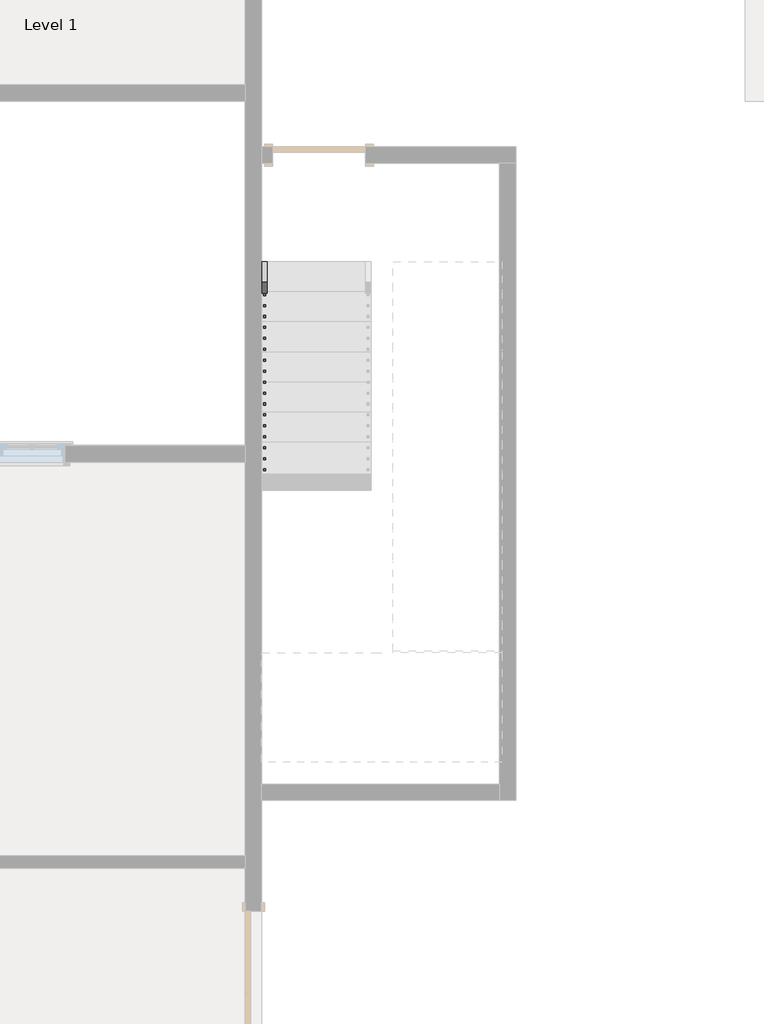
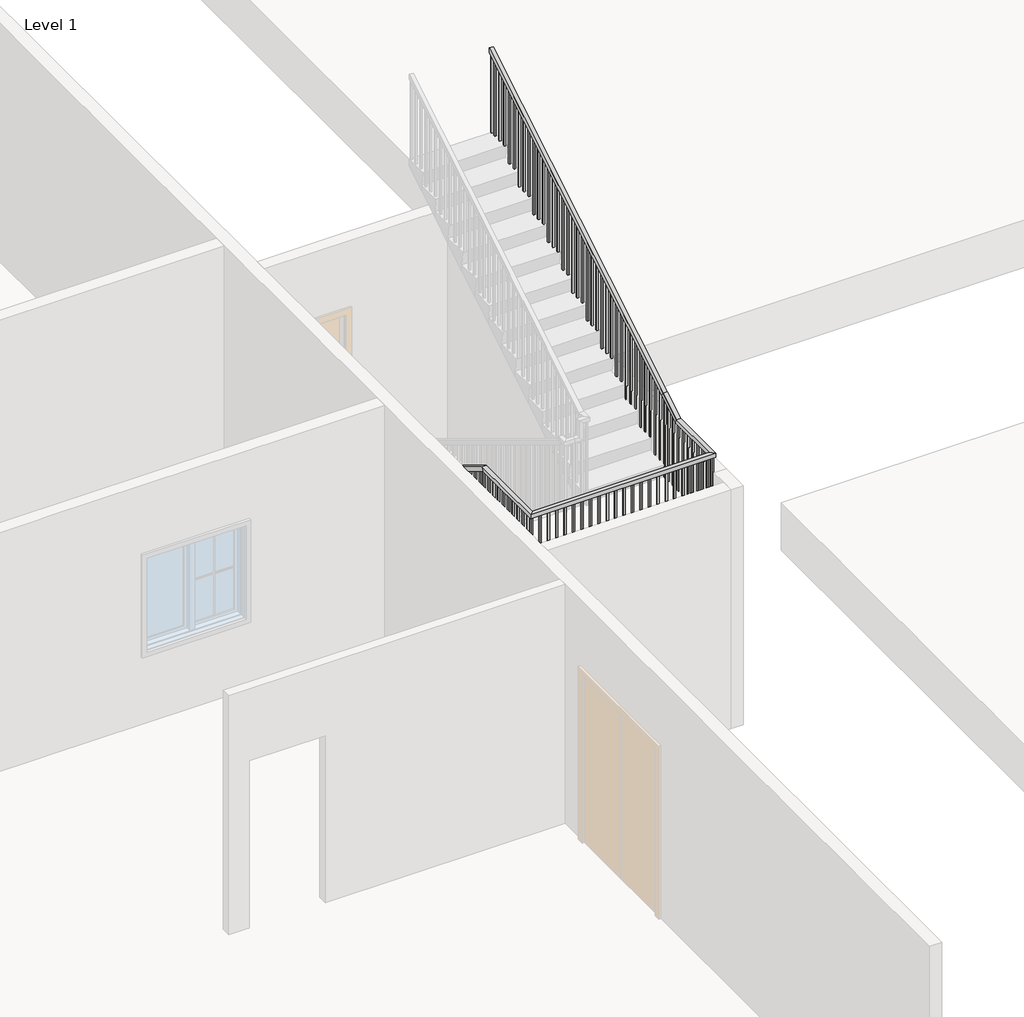
# One storey, part 4 of 7: 1 railing.
"""IFC4 building model written with IfcOpenShell, lengths in millimetres."""

from ifc_helpers import new_model, si_unit, frame, origin, place, context, project, spatial, polyline, outline, extrude, faceted_brep, element, save

model = new_model("IFC4")

# Units and contexts
model_context = context("Model", 3, world=origin())
ifc_project = project(units=[si_unit("LENGTHUNIT", "METRE", prefix="MILLI")], contexts=[model_context])

# Site, building, storey
site = spatial("IfcSite", under=ifc_project)
building = spatial("IfcBuilding", under=site)
storey = spatial("IfcBuildingStorey", under=building, Name="Level 1", Elevation=0.0)

# Railing
placement = place(None, origin())
element("IfcRailing", 1, ObjectType="Handrail - Rectangular", at=placement, inside=storey, context=model_context, shape_type="SolidModel", body=[
    faceted_brep([(-3452.3844485, 646.3269271, 1083.7333333), (-3452.3844485, 646.3269271, 1024.3318731), (-3503.1844485, 646.3269271, 1024.3318731), (-3503.1844485, 646.3269271, 1083.7333333), (-3452.3844485, -2985.8730729, 3285.0666667), (-3452.3844485, -3000.0654823, 3234.2666667), (-3503.1844485, -3000.0654823, 3234.2666667), (-3503.1844485, -2985.8730729, 3285.0666667), (-3452.3844485, -3951.0730729, 3285.0666667), (-3452.3844485, -3951.0730729, 3234.2666667), (-3503.1844485, -4001.8730729, 3234.2666667), (-3503.1844485, -4001.8730729, 3285.0666667), (-1318.7844485, -3951.0730729, 3285.0666667), (-1318.7844485, -3951.0730729, 3234.2666667), (-1267.9844485, -4001.8730729, 3234.2666667), (-1267.9844485, -4001.8730729, 3285.0666667), (-1318.7844485, -3265.2730729, 3285.0666667), (-1318.7844485, -3251.0806634, 3234.2666667), (-1267.9844485, -3251.0806634, 3234.2666667), (-1267.9844485, -3265.2730729, 3285.0666667), (-1318.7844485, -2985.8730729, 3454.4), (-1318.7844485, -2959.5433457, 3410.9559502), (-1267.9844485, -2959.5433457, 3410.9559502), (-1267.9844485, -2985.8730729, 3454.4), (-1318.7844485, 646.3269271, 5655.7333333), (-1267.9844485, 646.3269271, 5655.7333333), (-1267.9844485, 646.3269271, 5596.3318731), (-1318.7844485, 646.3269271, 5596.3318731)], [[[0, 1, 2, 3]], [[1, 0, 4, 5]], [[2, 1, 5, 6]], [[3, 2, 6, 7]], [[0, 3, 7, 4]], [[5, 4, 8, 9]], [[6, 5, 9, 10]], [[7, 6, 10, 11]], [[4, 7, 11, 8]], [[9, 8, 12, 13]], [[10, 9, 13, 14]], [[11, 10, 14, 15]], [[8, 11, 15, 12]], [[13, 12, 16, 17]], [[14, 13, 17, 18]], [[15, 14, 18, 19]], [[12, 15, 19, 16]], [[17, 16, 20, 21]], [[18, 17, 21, 22]], [[19, 18, 22, 23]], [[16, 19, 23, 20]], [[24, 25, 26, 27]], [[21, 20, 24, 27]], [[22, 21, 27, 26]], [[23, 22, 26, 25]], [[20, 23, 25, 24]]]),
    extrude(outline(polyline([(560.6019271, 5544.3773276), (579.6519271, 5555.9227822), (579.6519271, 4572.0), (560.6019271, 4572.0), (560.6019271, 5544.3773276)])), frame((-1302.9094485, 0.0, 0.0), z_axis=(1.0, 0.0, 0.0), x_axis=(0.0, 1.0, 0.0)), (0.0, 0.0, 1.0), 19.05),
    extrude(outline(polyline([(459.0019271, 5482.80157), (478.0519271, 5494.3470246), (478.0519271, 4572.0), (459.0019271, 4572.0), (459.0019271, 5482.80157)])), frame((-1302.9094485, 0.0, 0.0), z_axis=(1.0, 0.0, 0.0), x_axis=(0.0, 1.0, 0.0)), (0.0, 0.0, 1.0), 19.05),
    extrude(outline(polyline([(357.4019271, 5421.2258125), (376.4519271, 5432.771267), (376.4519271, 4572.0), (357.4019271, 4572.0), (357.4019271, 5421.2258125)])), frame((-1302.9094485, 0.0, 0.0), z_axis=(1.0, 0.0, 0.0), x_axis=(0.0, 1.0, 0.0)), (0.0, 0.0, 1.0), 19.05),
    extrude(outline(polyline([(255.8019271, 5359.6500549), (274.8519271, 5371.1955094), (274.8519271, 4402.6666667), (255.8019271, 4402.6666667), (255.8019271, 5359.6500549)])), frame((-1302.9094485, 0.0, 0.0), z_axis=(1.0, 0.0, 0.0), x_axis=(0.0, 1.0, 0.0)), (0.0, 0.0, 1.0), 19.05),
    extrude(outline(polyline([(154.2019271, 5298.0742973), (173.2519271, 5309.6197519), (173.2519271, 4402.6666667), (154.2019271, 4402.6666667), (154.2019271, 5298.0742973)])), frame((-1302.9094485, 0.0, 0.0), z_axis=(1.0, 0.0, 0.0), x_axis=(0.0, 1.0, 0.0)), (0.0, 0.0, 1.0), 19.05),
    extrude(outline(polyline([(52.6019271, 5236.4985397), (71.6519271, 5248.0439943), (71.6519271, 4233.3333333), (52.6019271, 4233.3333333), (52.6019271, 5236.4985397)])), frame((-1302.9094485, 0.0, 0.0), z_axis=(1.0, 0.0, 0.0), x_axis=(0.0, 1.0, 0.0)), (0.0, 0.0, 1.0), 19.05),
    extrude(outline(polyline([(-48.9980729, 5174.9227822), (-29.9480729, 5186.4682367), (-29.9480729, 4233.3333333), (-48.9980729, 4233.3333333), (-48.9980729, 5174.9227822)])), frame((-1302.9094485, 0.0, 0.0), z_axis=(1.0, 0.0, 0.0), x_axis=(0.0, 1.0, 0.0)), (0.0, 0.0, 1.0), 19.05),
    extrude(outline(polyline([(-150.5980729, 5113.3470246), (-131.5480729, 5124.8924791), (-131.5480729, 4233.3333333), (-150.5980729, 4233.3333333), (-150.5980729, 5113.3470246)])), frame((-1302.9094485, 0.0, 0.0), z_axis=(1.0, 0.0, 0.0), x_axis=(0.0, 1.0, 0.0)), (0.0, 0.0, 1.0), 19.05),
    extrude(outline(polyline([(-252.1980729, 5051.771267), (-233.1480729, 5063.3167216), (-233.1480729, 4064.0), (-252.1980729, 4064.0), (-252.1980729, 5051.771267)])), frame((-1302.9094485, 0.0, 0.0), z_axis=(1.0, 0.0, 0.0), x_axis=(0.0, 1.0, 0.0)), (0.0, 0.0, 1.0), 19.05),
    extrude(outline(polyline([(-353.7980729, 4990.1955094), (-334.7480729, 5001.740964), (-334.7480729, 4064.0), (-353.7980729, 4064.0), (-353.7980729, 4990.1955094)])), frame((-1302.9094485, 0.0, 0.0), z_axis=(1.0, 0.0, 0.0), x_axis=(0.0, 1.0, 0.0)), (0.0, 0.0, 1.0), 19.05),
    extrude(outline(polyline([(-455.3980729, 4928.6197519), (-436.3480729, 4940.1652064), (-436.3480729, 4064.0), (-455.3980729, 4064.0), (-455.3980729, 4928.6197519)])), frame((-1302.9094485, 0.0, 0.0), z_axis=(1.0, 0.0, 0.0), x_axis=(0.0, 1.0, 0.0)), (0.0, 0.0, 1.0), 19.05),
    extrude(outline(polyline([(-556.9980729, 4867.0439943), (-537.9480729, 4878.5894488), (-537.9480729, 3894.6666667), (-556.9980729, 3894.6666667), (-556.9980729, 4867.0439943)])), frame((-1302.9094485, 0.0, 0.0), z_axis=(1.0, 0.0, 0.0), x_axis=(0.0, 1.0, 0.0)), (0.0, 0.0, 1.0), 19.05),
    extrude(outline(polyline([(-658.5980729, 4805.4682367), (-639.5480729, 4817.0136913), (-639.5480729, 3894.6666667), (-658.5980729, 3894.6666667), (-658.5980729, 4805.4682367)])), frame((-1302.9094485, 0.0, 0.0), z_axis=(1.0, 0.0, 0.0), x_axis=(0.0, 1.0, 0.0)), (0.0, 0.0, 1.0), 19.05),
    extrude(outline(polyline([(-760.1980729, 4743.8924791), (-741.1480729, 4755.4379337), (-741.1480729, 3894.6666667), (-760.1980729, 3894.6666667), (-760.1980729, 4743.8924791)])), frame((-1302.9094485, 0.0, 0.0), z_axis=(1.0, 0.0, 0.0), x_axis=(0.0, 1.0, 0.0)), (0.0, 0.0, 1.0), 19.05),
    extrude(outline(polyline([(-861.7980729, 4682.3167216), (-842.7480729, 4693.8621761), (-842.7480729, 3725.3333333), (-861.7980729, 3725.3333333), (-861.7980729, 4682.3167216)])), frame((-1302.9094485, 0.0, 0.0), z_axis=(1.0, 0.0, 0.0), x_axis=(0.0, 1.0, 0.0)), (0.0, 0.0, 1.0), 19.05),
    extrude(outline(polyline([(-963.3980729, 4620.740964), (-944.3480729, 4632.2864185), (-944.3480729, 3725.3333333), (-963.3980729, 3725.3333333), (-963.3980729, 4620.740964)])), frame((-1302.9094485, 0.0, 0.0), z_axis=(1.0, 0.0, 0.0), x_axis=(0.0, 1.0, 0.0)), (0.0, 0.0, 1.0), 19.05),
    extrude(outline(polyline([(-1064.9980729, 4559.1652064), (-1045.9480729, 4570.710661), (-1045.9480729, 3556.0), (-1064.9980729, 3556.0), (-1064.9980729, 4559.1652064)])), frame((-1302.9094485, 0.0, 0.0), z_axis=(1.0, 0.0, 0.0), x_axis=(0.0, 1.0, 0.0)), (0.0, 0.0, 1.0), 19.05),
    extrude(outline(polyline([(-1166.5980729, 4497.5894488), (-1147.5480729, 4509.1349034), (-1147.5480729, 3556.0), (-1166.5980729, 3556.0), (-1166.5980729, 4497.5894488)])), frame((-1302.9094485, 0.0, 0.0), z_axis=(1.0, 0.0, 0.0), x_axis=(0.0, 1.0, 0.0)), (0.0, 0.0, 1.0), 19.05),
    extrude(outline(polyline([(-1268.1980729, 4436.0136913), (-1249.1480729, 4447.5591458), (-1249.1480729, 3556.0), (-1268.1980729, 3556.0), (-1268.1980729, 4436.0136913)])), frame((-1302.9094485, 0.0, 0.0), z_axis=(1.0, 0.0, 0.0), x_axis=(0.0, 1.0, 0.0)), (0.0, 0.0, 1.0), 19.05),
    extrude(outline(polyline([(-1369.7980729, 4374.4379337), (-1350.7480729, 4385.9833882), (-1350.7480729, 3386.6666667), (-1369.7980729, 3386.6666667), (-1369.7980729, 4374.4379337)])), frame((-1302.9094485, 0.0, 0.0), z_axis=(1.0, 0.0, 0.0), x_axis=(0.0, 1.0, 0.0)), (0.0, 0.0, 1.0), 19.05),
    extrude(outline(polyline([(-1471.3980729, 4312.8621761), (-1452.3480729, 4324.4076307), (-1452.3480729, 3386.6666667), (-1471.3980729, 3386.6666667), (-1471.3980729, 4312.8621761)])), frame((-1302.9094485, 0.0, 0.0), z_axis=(1.0, 0.0, 0.0), x_axis=(0.0, 1.0, 0.0)), (0.0, 0.0, 1.0), 19.05),
    extrude(outline(polyline([(-1572.9980729, 4251.2864185), (-1553.9480729, 4262.8318731), (-1553.9480729, 3386.6666667), (-1572.9980729, 3386.6666667), (-1572.9980729, 4251.2864185)])), frame((-1302.9094485, 0.0, 0.0), z_axis=(1.0, 0.0, 0.0), x_axis=(0.0, 1.0, 0.0)), (0.0, 0.0, 1.0), 19.05),
    extrude(outline(polyline([(-1674.5980729, 4189.710661), (-1655.5480729, 4201.2561155), (-1655.5480729, 3217.3333333), (-1674.5980729, 3217.3333333), (-1674.5980729, 4189.710661)])), frame((-1302.9094485, 0.0, 0.0), z_axis=(1.0, 0.0, 0.0), x_axis=(0.0, 1.0, 0.0)), (0.0, 0.0, 1.0), 19.05),
    extrude(outline(polyline([(-1776.1980729, 4128.1349034), (-1757.1480729, 4139.6803579), (-1757.1480729, 3217.3333333), (-1776.1980729, 3217.3333333), (-1776.1980729, 4128.1349034)])), frame((-1302.9094485, 0.0, 0.0), z_axis=(1.0, 0.0, 0.0), x_axis=(0.0, 1.0, 0.0)), (0.0, 0.0, 1.0), 19.05),
    extrude(outline(polyline([(-1877.7980729, 4066.5591458), (-1858.7480729, 4078.1046004), (-1858.7480729, 3217.3333333), (-1877.7980729, 3217.3333333), (-1877.7980729, 4066.5591458)])), frame((-1302.9094485, 0.0, 0.0), z_axis=(1.0, 0.0, 0.0), x_axis=(0.0, 1.0, 0.0)), (0.0, 0.0, 1.0), 19.05),
    extrude(outline(polyline([(-1979.3980729, 4004.9833882), (-1960.3480729, 4016.5288428), (-1960.3480729, 3048.0), (-1979.3980729, 3048.0), (-1979.3980729, 4004.9833882)])), frame((-1302.9094485, 0.0, 0.0), z_axis=(1.0, 0.0, 0.0), x_axis=(0.0, 1.0, 0.0)), (0.0, 0.0, 1.0), 19.05),
    extrude(outline(polyline([(-2080.9980729, 3943.4076307), (-2061.9480729, 3954.9530852), (-2061.9480729, 3048.0), (-2080.9980729, 3048.0), (-2080.9980729, 3943.4076307)])), frame((-1302.9094485, 0.0, 0.0), z_axis=(1.0, 0.0, 0.0), x_axis=(0.0, 1.0, 0.0)), (0.0, 0.0, 1.0), 19.05),
    extrude(outline(polyline([(-2182.5980729, 3881.8318731), (-2163.5480729, 3893.3773276), (-2163.5480729, 2878.6666667), (-2182.5980729, 2878.6666667), (-2182.5980729, 3881.8318731)])), frame((-1302.9094485, 0.0, 0.0), z_axis=(1.0, 0.0, 0.0), x_axis=(0.0, 1.0, 0.0)), (0.0, 0.0, 1.0), 19.05),
    extrude(outline(polyline([(-2284.1980729, 3820.2561155), (-2265.1480729, 3831.80157), (-2265.1480729, 2878.6666667), (-2284.1980729, 2878.6666667), (-2284.1980729, 3820.2561155)])), frame((-1302.9094485, 0.0, 0.0), z_axis=(1.0, 0.0, 0.0), x_axis=(0.0, 1.0, 0.0)), (0.0, 0.0, 1.0), 19.05),
    extrude(outline(polyline([(-2385.7980729, 3758.6803579), (-2366.7480729, 3770.2258125), (-2366.7480729, 2878.6666667), (-2385.7980729, 2878.6666667), (-2385.7980729, 3758.6803579)])), frame((-1302.9094485, 0.0, 0.0), z_axis=(1.0, 0.0, 0.0), x_axis=(0.0, 1.0, 0.0)), (0.0, 0.0, 1.0), 19.05),
    extrude(outline(polyline([(-2487.3980729, 3697.1046004), (-2468.3480729, 3708.6500549), (-2468.3480729, 2709.3333333), (-2487.3980729, 2709.3333333), (-2487.3980729, 3697.1046004)])), frame((-1302.9094485, 0.0, 0.0), z_axis=(1.0, 0.0, 0.0), x_axis=(0.0, 1.0, 0.0)), (0.0, 0.0, 1.0), 19.05),
    extrude(outline(polyline([(-2588.9980729, 3635.5288428), (-2569.9480729, 3647.0742973), (-2569.9480729, 2709.3333333), (-2588.9980729, 2709.3333333), (-2588.9980729, 3635.5288428)])), frame((-1302.9094485, 0.0, 0.0), z_axis=(1.0, 0.0, 0.0), x_axis=(0.0, 1.0, 0.0)), (0.0, 0.0, 1.0), 19.05),
    extrude(outline(polyline([(-2690.5980729, 3573.9530852), (-2671.5480729, 3585.4985397), (-2671.5480729, 2709.3333333), (-2690.5980729, 2709.3333333), (-2690.5980729, 3573.9530852)])), frame((-1302.9094485, 0.0, 0.0), z_axis=(1.0, 0.0, 0.0), x_axis=(0.0, 1.0, 0.0)), (0.0, 0.0, 1.0), 19.05),
    extrude(outline(polyline([(-2792.1980729, 3512.3773276), (-2773.1480729, 3523.9227822), (-2773.1480729, 2540.0), (-2792.1980729, 2540.0), (-2792.1980729, 3512.3773276)])), frame((-1302.9094485, 0.0, 0.0), z_axis=(1.0, 0.0, 0.0), x_axis=(0.0, 1.0, 0.0)), (0.0, 0.0, 1.0), 19.05),
    extrude(outline(polyline([(-2893.7980729, 3450.80157), (-2874.7480729, 3462.3470246), (-2874.7480729, 2540.0), (-2893.7980729, 2540.0), (-2893.7980729, 3450.80157)])), frame((-1302.9094485, 0.0, 0.0), z_axis=(1.0, 0.0, 0.0), x_axis=(0.0, 1.0, 0.0)), (0.0, 0.0, 1.0), 19.05),
    extrude(outline(polyline([(-3071.5980729, 3343.0439943), (-3052.5480729, 3354.5894488), (-3052.5480729, 2370.6666667), (-3071.5980729, 2370.6666667), (-3071.5980729, 3343.0439943)])), frame((-1302.9094485, 0.0, 0.0), z_axis=(1.0, 0.0, 0.0), x_axis=(0.0, 1.0, 0.0)), (0.0, 0.0, 1.0), 19.05),
    extrude(outline(polyline([(-3173.1980729, 3281.4682367), (-3154.1480729, 3293.0136913), (-3154.1480729, 2370.6666667), (-3173.1980729, 2370.6666667), (-3173.1980729, 3281.4682367)])), frame((-1302.9094485, 0.0, 0.0), z_axis=(1.0, 0.0, 0.0), x_axis=(0.0, 1.0, 0.0)), (0.0, 0.0, 1.0), 19.05),
    extrude(outline(polyline([(-1283.8594485, -3274.7980729), (-1302.9094485, -3274.7980729), (-1302.9094485, -3255.7480729), (-1283.8594485, -3255.7480729), (-1283.8594485, -3274.7980729)])), frame((0.0, 0.0, 2370.6666667), z_axis=(0.0, 0.0, 1.0), x_axis=(1.0, 0.0, 0.0)), (0.0, 0.0, 1.0), 863.6),
    extrude(outline(polyline([(-1283.8594485, -3376.3980729), (-1302.9094485, -3376.3980729), (-1302.9094485, -3357.3480729), (-1283.8594485, -3357.3480729), (-1283.8594485, -3376.3980729)])), frame((0.0, 0.0, 2370.6666667), z_axis=(0.0, 0.0, 1.0), x_axis=(1.0, 0.0, 0.0)), (0.0, 0.0, 1.0), 863.6),
    extrude(outline(polyline([(-1283.8594485, -3477.9980729), (-1302.9094485, -3477.9980729), (-1302.9094485, -3458.9480729), (-1283.8594485, -3458.9480729), (-1283.8594485, -3477.9980729)])), frame((0.0, 0.0, 2370.6666667), z_axis=(0.0, 0.0, 1.0), x_axis=(1.0, 0.0, 0.0)), (0.0, 0.0, 1.0), 863.6),
    extrude(outline(polyline([(-1283.8594485, -3579.5980729), (-1302.9094485, -3579.5980729), (-1302.9094485, -3560.5480729), (-1283.8594485, -3560.5480729), (-1283.8594485, -3579.5980729)])), frame((0.0, 0.0, 2370.6666667), z_axis=(0.0, 0.0, 1.0), x_axis=(1.0, 0.0, 0.0)), (0.0, 0.0, 1.0), 863.6),
    extrude(outline(polyline([(-1283.8594485, -3681.1980729), (-1302.9094485, -3681.1980729), (-1302.9094485, -3662.1480729), (-1283.8594485, -3662.1480729), (-1283.8594485, -3681.1980729)])), frame((0.0, 0.0, 2370.6666667), z_axis=(0.0, 0.0, 1.0), x_axis=(1.0, 0.0, 0.0)), (0.0, 0.0, 1.0), 863.6),
    extrude(outline(polyline([(-1283.8594485, -3782.7980729), (-1302.9094485, -3782.7980729), (-1302.9094485, -3763.7480729), (-1283.8594485, -3763.7480729), (-1283.8594485, -3782.7980729)])), frame((0.0, 0.0, 2370.6666667), z_axis=(0.0, 0.0, 1.0), x_axis=(1.0, 0.0, 0.0)), (0.0, 0.0, 1.0), 863.6),
    extrude(outline(polyline([(-1283.8594485, -3884.3980729), (-1302.9094485, -3884.3980729), (-1302.9094485, -3865.3480729), (-1283.8594485, -3865.3480729), (-1283.8594485, -3884.3980729)])), frame((0.0, 0.0, 2370.6666667), z_axis=(0.0, 0.0, 1.0), x_axis=(1.0, 0.0, 0.0)), (0.0, 0.0, 1.0), 863.6),
    extrude(outline(polyline([(-1353.7094485, -3985.9980729), (-1353.7094485, -3966.9480729), (-1334.6594485, -3966.9480729), (-1334.6594485, -3985.9980729), (-1353.7094485, -3985.9980729)])), frame((0.0, 0.0, 2370.6666667), z_axis=(0.0, 0.0, 1.0), x_axis=(1.0, 0.0, 0.0)), (0.0, 0.0, 1.0), 863.6),
    extrude(outline(polyline([(-1455.3094485, -3985.9980729), (-1455.3094485, -3966.9480729), (-1436.2594485, -3966.9480729), (-1436.2594485, -3985.9980729), (-1455.3094485, -3985.9980729)])), frame((0.0, 0.0, 2370.6666667), z_axis=(0.0, 0.0, 1.0), x_axis=(1.0, 0.0, 0.0)), (0.0, 0.0, 1.0), 863.6),
    extrude(outline(polyline([(-1556.9094485, -3985.9980729), (-1556.9094485, -3966.9480729), (-1537.8594485, -3966.9480729), (-1537.8594485, -3985.9980729), (-1556.9094485, -3985.9980729)])), frame((0.0, 0.0, 2370.6666667), z_axis=(0.0, 0.0, 1.0), x_axis=(1.0, 0.0, 0.0)), (0.0, 0.0, 1.0), 863.6),
    extrude(outline(polyline([(-1658.5094485, -3985.9980729), (-1658.5094485, -3966.9480729), (-1639.4594485, -3966.9480729), (-1639.4594485, -3985.9980729), (-1658.5094485, -3985.9980729)])), frame((0.0, 0.0, 2370.6666667), z_axis=(0.0, 0.0, 1.0), x_axis=(1.0, 0.0, 0.0)), (0.0, 0.0, 1.0), 863.6),
    extrude(outline(polyline([(-1760.1094485, -3985.9980729), (-1760.1094485, -3966.9480729), (-1741.0594485, -3966.9480729), (-1741.0594485, -3985.9980729), (-1760.1094485, -3985.9980729)])), frame((0.0, 0.0, 2370.6666667), z_axis=(0.0, 0.0, 1.0), x_axis=(1.0, 0.0, 0.0)), (0.0, 0.0, 1.0), 863.6),
    extrude(outline(polyline([(-1861.7094485, -3985.9980729), (-1861.7094485, -3966.9480729), (-1842.6594485, -3966.9480729), (-1842.6594485, -3985.9980729), (-1861.7094485, -3985.9980729)])), frame((0.0, 0.0, 2370.6666667), z_axis=(0.0, 0.0, 1.0), x_axis=(1.0, 0.0, 0.0)), (0.0, 0.0, 1.0), 863.6),
    extrude(outline(polyline([(-1963.3094485, -3985.9980729), (-1963.3094485, -3966.9480729), (-1944.2594485, -3966.9480729), (-1944.2594485, -3985.9980729), (-1963.3094485, -3985.9980729)])), frame((0.0, 0.0, 2370.6666667), z_axis=(0.0, 0.0, 1.0), x_axis=(1.0, 0.0, 0.0)), (0.0, 0.0, 1.0), 863.6),
    extrude(outline(polyline([(-2064.9094485, -3985.9980729), (-2064.9094485, -3966.9480729), (-2045.8594485, -3966.9480729), (-2045.8594485, -3985.9980729), (-2064.9094485, -3985.9980729)])), frame((0.0, 0.0, 2370.6666667), z_axis=(0.0, 0.0, 1.0), x_axis=(1.0, 0.0, 0.0)), (0.0, 0.0, 1.0), 863.6),
    extrude(outline(polyline([(-2166.5094485, -3985.9980729), (-2166.5094485, -3966.9480729), (-2147.4594485, -3966.9480729), (-2147.4594485, -3985.9980729), (-2166.5094485, -3985.9980729)])), frame((0.0, 0.0, 2370.6666667), z_axis=(0.0, 0.0, 1.0), x_axis=(1.0, 0.0, 0.0)), (0.0, 0.0, 1.0), 863.6),
    extrude(outline(polyline([(-2268.1094485, -3985.9980729), (-2268.1094485, -3966.9480729), (-2249.0594485, -3966.9480729), (-2249.0594485, -3985.9980729), (-2268.1094485, -3985.9980729)])), frame((0.0, 0.0, 2370.6666667), z_axis=(0.0, 0.0, 1.0), x_axis=(1.0, 0.0, 0.0)), (0.0, 0.0, 1.0), 863.6),
    extrude(outline(polyline([(-2369.7094485, -3985.9980729), (-2369.7094485, -3966.9480729), (-2350.6594485, -3966.9480729), (-2350.6594485, -3985.9980729), (-2369.7094485, -3985.9980729)])), frame((0.0, 0.0, 2370.6666667), z_axis=(0.0, 0.0, 1.0), x_axis=(1.0, 0.0, 0.0)), (0.0, 0.0, 1.0), 863.6),
    extrude(outline(polyline([(-2471.3094485, -3985.9980729), (-2471.3094485, -3966.9480729), (-2452.2594485, -3966.9480729), (-2452.2594485, -3985.9980729), (-2471.3094485, -3985.9980729)])), frame((0.0, 0.0, 2370.6666667), z_axis=(0.0, 0.0, 1.0), x_axis=(1.0, 0.0, 0.0)), (0.0, 0.0, 1.0), 863.6),
    extrude(outline(polyline([(-2572.9094485, -3985.9980729), (-2572.9094485, -3966.9480729), (-2553.8594485, -3966.9480729), (-2553.8594485, -3985.9980729), (-2572.9094485, -3985.9980729)])), frame((0.0, 0.0, 2370.6666667), z_axis=(0.0, 0.0, 1.0), x_axis=(1.0, 0.0, 0.0)), (0.0, 0.0, 1.0), 863.6),
    extrude(outline(polyline([(-2674.5094485, -3985.9980729), (-2674.5094485, -3966.9480729), (-2655.4594485, -3966.9480729), (-2655.4594485, -3985.9980729), (-2674.5094485, -3985.9980729)])), frame((0.0, 0.0, 2370.6666667), z_axis=(0.0, 0.0, 1.0), x_axis=(1.0, 0.0, 0.0)), (0.0, 0.0, 1.0), 863.6),
    extrude(outline(polyline([(-2776.1094485, -3985.9980729), (-2776.1094485, -3966.9480729), (-2757.0594485, -3966.9480729), (-2757.0594485, -3985.9980729), (-2776.1094485, -3985.9980729)])), frame((0.0, 0.0, 2370.6666667), z_axis=(0.0, 0.0, 1.0), x_axis=(1.0, 0.0, 0.0)), (0.0, 0.0, 1.0), 863.6),
    extrude(outline(polyline([(-2877.7094485, -3985.9980729), (-2877.7094485, -3966.9480729), (-2858.6594485, -3966.9480729), (-2858.6594485, -3985.9980729), (-2877.7094485, -3985.9980729)])), frame((0.0, 0.0, 2370.6666667), z_axis=(0.0, 0.0, 1.0), x_axis=(1.0, 0.0, 0.0)), (0.0, 0.0, 1.0), 863.6),
    extrude(outline(polyline([(-2979.3094485, -3985.9980729), (-2979.3094485, -3966.9480729), (-2960.2594485, -3966.9480729), (-2960.2594485, -3985.9980729), (-2979.3094485, -3985.9980729)])), frame((0.0, 0.0, 2370.6666667), z_axis=(0.0, 0.0, 1.0), x_axis=(1.0, 0.0, 0.0)), (0.0, 0.0, 1.0), 863.6),
    extrude(outline(polyline([(-3080.9094485, -3985.9980729), (-3080.9094485, -3966.9480729), (-3061.8594485, -3966.9480729), (-3061.8594485, -3985.9980729), (-3080.9094485, -3985.9980729)])), frame((0.0, 0.0, 2370.6666667), z_axis=(0.0, 0.0, 1.0), x_axis=(1.0, 0.0, 0.0)), (0.0, 0.0, 1.0), 863.6),
    extrude(outline(polyline([(-3182.5094485, -3985.9980729), (-3182.5094485, -3966.9480729), (-3163.4594485, -3966.9480729), (-3163.4594485, -3985.9980729), (-3182.5094485, -3985.9980729)])), frame((0.0, 0.0, 2370.6666667), z_axis=(0.0, 0.0, 1.0), x_axis=(1.0, 0.0, 0.0)), (0.0, 0.0, 1.0), 863.6),
    extrude(outline(polyline([(-3284.1094485, -3985.9980729), (-3284.1094485, -3966.9480729), (-3265.0594485, -3966.9480729), (-3265.0594485, -3985.9980729), (-3284.1094485, -3985.9980729)])), frame((0.0, 0.0, 2370.6666667), z_axis=(0.0, 0.0, 1.0), x_axis=(1.0, 0.0, 0.0)), (0.0, 0.0, 1.0), 863.6),
    extrude(outline(polyline([(-3385.7094485, -3985.9980729), (-3385.7094485, -3966.9480729), (-3366.6594485, -3966.9480729), (-3366.6594485, -3985.9980729), (-3385.7094485, -3985.9980729)])), frame((0.0, 0.0, 2370.6666667), z_axis=(0.0, 0.0, 1.0), x_axis=(1.0, 0.0, 0.0)), (0.0, 0.0, 1.0), 863.6),
    extrude(outline(polyline([(-3487.3094485, -3890.7480729), (-3468.2594485, -3890.7480729), (-3468.2594485, -3909.7980729), (-3487.3094485, -3909.7980729), (-3487.3094485, -3890.7480729)])), frame((0.0, 0.0, 2370.6666667), z_axis=(0.0, 0.0, 1.0), x_axis=(1.0, 0.0, 0.0)), (0.0, 0.0, 1.0), 863.6),
    extrude(outline(polyline([(-3487.3094485, -3789.1480729), (-3468.2594485, -3789.1480729), (-3468.2594485, -3808.1980729), (-3487.3094485, -3808.1980729), (-3487.3094485, -3789.1480729)])), frame((0.0, 0.0, 2370.6666667), z_axis=(0.0, 0.0, 1.0), x_axis=(1.0, 0.0, 0.0)), (0.0, 0.0, 1.0), 863.6),
    extrude(outline(polyline([(-3487.3094485, -3687.5480729), (-3468.2594485, -3687.5480729), (-3468.2594485, -3706.5980729), (-3487.3094485, -3706.5980729), (-3487.3094485, -3687.5480729)])), frame((0.0, 0.0, 2370.6666667), z_axis=(0.0, 0.0, 1.0), x_axis=(1.0, 0.0, 0.0)), (0.0, 0.0, 1.0), 863.6),
    extrude(outline(polyline([(-3487.3094485, -3585.9480729), (-3468.2594485, -3585.9480729), (-3468.2594485, -3604.9980729), (-3487.3094485, -3604.9980729), (-3487.3094485, -3585.9480729)])), frame((0.0, 0.0, 2370.6666667), z_axis=(0.0, 0.0, 1.0), x_axis=(1.0, 0.0, 0.0)), (0.0, 0.0, 1.0), 863.6),
    extrude(outline(polyline([(-3487.3094485, -3484.3480729), (-3468.2594485, -3484.3480729), (-3468.2594485, -3503.3980729), (-3487.3094485, -3503.3980729), (-3487.3094485, -3484.3480729)])), frame((0.0, 0.0, 2370.6666667), z_axis=(0.0, 0.0, 1.0), x_axis=(1.0, 0.0, 0.0)), (0.0, 0.0, 1.0), 863.6),
    extrude(outline(polyline([(-3487.3094485, -3382.7480729), (-3468.2594485, -3382.7480729), (-3468.2594485, -3401.7980729), (-3487.3094485, -3401.7980729), (-3487.3094485, -3382.7480729)])), frame((0.0, 0.0, 2370.6666667), z_axis=(0.0, 0.0, 1.0), x_axis=(1.0, 0.0, 0.0)), (0.0, 0.0, 1.0), 863.6),
    extrude(outline(polyline([(-3487.3094485, -3281.1480729), (-3468.2594485, -3281.1480729), (-3468.2594485, -3300.1980729), (-3487.3094485, -3300.1980729), (-3487.3094485, -3281.1480729)])), frame((0.0, 0.0, 2370.6666667), z_axis=(0.0, 0.0, 1.0), x_axis=(1.0, 0.0, 0.0)), (0.0, 0.0, 1.0), 863.6),
    extrude(outline(polyline([(-3487.3094485, -3179.5480729), (-3468.2594485, -3179.5480729), (-3468.2594485, -3198.5980729), (-3487.3094485, -3198.5980729), (-3487.3094485, -3179.5480729)])), frame((0.0, 0.0, 2370.6666667), z_axis=(0.0, 0.0, 1.0), x_axis=(1.0, 0.0, 0.0)), (0.0, 0.0, 1.0), 863.6),
    extrude(outline(polyline([(-3487.3094485, -3077.9480729), (-3468.2594485, -3077.9480729), (-3468.2594485, -3096.9980729), (-3487.3094485, -3096.9980729), (-3487.3094485, -3077.9480729)])), frame((0.0, 0.0, 2370.6666667), z_axis=(0.0, 0.0, 1.0), x_axis=(1.0, 0.0, 0.0)), (0.0, 0.0, 1.0), 863.6),
    extrude(outline(polyline([(-2919.1980729, 3185.2561155), (-2900.1480729, 3173.710661), (-2900.1480729, 2201.3333333), (-2919.1980729, 2201.3333333), (-2919.1980729, 3185.2561155)])), frame((-3487.3094485, 0.0, 0.0), z_axis=(1.0, 0.0, 0.0), x_axis=(0.0, 1.0, 0.0)), (0.0, 0.0, 1.0), 19.05),
    extrude(outline(polyline([(-2817.5980729, 3123.6803579), (-2798.5480729, 3112.1349034), (-2798.5480729, 2201.3333333), (-2817.5980729, 2201.3333333), (-2817.5980729, 3123.6803579)])), frame((-3487.3094485, 0.0, 0.0), z_axis=(1.0, 0.0, 0.0), x_axis=(0.0, 1.0, 0.0)), (0.0, 0.0, 1.0), 19.05),
    extrude(outline(polyline([(-2715.9980729, 3062.1046004), (-2696.9480729, 3050.5591458), (-2696.9480729, 2201.3333333), (-2715.9980729, 2201.3333333), (-2715.9980729, 3062.1046004)])), frame((-3487.3094485, 0.0, 0.0), z_axis=(1.0, 0.0, 0.0), x_axis=(0.0, 1.0, 0.0)), (0.0, 0.0, 1.0), 19.05),
    extrude(outline(polyline([(-2614.3980729, 3000.5288428), (-2595.3480729, 2988.9833882), (-2595.3480729, 2032.0), (-2614.3980729, 2032.0), (-2614.3980729, 3000.5288428)])), frame((-3487.3094485, 0.0, 0.0), z_axis=(1.0, 0.0, 0.0), x_axis=(0.0, 1.0, 0.0)), (0.0, 0.0, 1.0), 19.05),
    extrude(outline(polyline([(-2512.7980729, 2938.9530852), (-2493.7480729, 2927.4076307), (-2493.7480729, 2032.0), (-2512.7980729, 2032.0), (-2512.7980729, 2938.9530852)])), frame((-3487.3094485, 0.0, 0.0), z_axis=(1.0, 0.0, 0.0), x_axis=(0.0, 1.0, 0.0)), (0.0, 0.0, 1.0), 19.05),
    extrude(outline(polyline([(-2411.1980729, 2877.3773276), (-2392.1480729, 2865.8318731), (-2392.1480729, 1862.6666667), (-2411.1980729, 1862.6666667), (-2411.1980729, 2877.3773276)])), frame((-3487.3094485, 0.0, 0.0), z_axis=(1.0, 0.0, 0.0), x_axis=(0.0, 1.0, 0.0)), (0.0, 0.0, 1.0), 19.05),
    extrude(outline(polyline([(-2309.5980729, 2815.80157), (-2290.5480729, 2804.2561155), (-2290.5480729, 1862.6666667), (-2309.5980729, 1862.6666667), (-2309.5980729, 2815.80157)])), frame((-3487.3094485, 0.0, 0.0), z_axis=(1.0, 0.0, 0.0), x_axis=(0.0, 1.0, 0.0)), (0.0, 0.0, 1.0), 19.05),
    extrude(outline(polyline([(-2207.9980729, 2754.2258125), (-2188.9480729, 2742.6803579), (-2188.9480729, 1862.6666667), (-2207.9980729, 1862.6666667), (-2207.9980729, 2754.2258125)])), frame((-3487.3094485, 0.0, 0.0), z_axis=(1.0, 0.0, 0.0), x_axis=(0.0, 1.0, 0.0)), (0.0, 0.0, 1.0), 19.05),
    extrude(outline(polyline([(-2106.3980729, 2692.6500549), (-2087.3480729, 2681.1046004), (-2087.3480729, 1693.3333333), (-2106.3980729, 1693.3333333), (-2106.3980729, 2692.6500549)])), frame((-3487.3094485, 0.0, 0.0), z_axis=(1.0, 0.0, 0.0), x_axis=(0.0, 1.0, 0.0)), (0.0, 0.0, 1.0), 19.05),
    extrude(outline(polyline([(-2004.7980729, 2631.0742973), (-1985.7480729, 2619.5288428), (-1985.7480729, 1693.3333333), (-2004.7980729, 1693.3333333), (-2004.7980729, 2631.0742973)])), frame((-3487.3094485, 0.0, 0.0), z_axis=(1.0, 0.0, 0.0), x_axis=(0.0, 1.0, 0.0)), (0.0, 0.0, 1.0), 19.05),
    extrude(outline(polyline([(-1903.1980729, 2569.4985397), (-1884.1480729, 2557.9530852), (-1884.1480729, 1693.3333333), (-1903.1980729, 1693.3333333), (-1903.1980729, 2569.4985397)])), frame((-3487.3094485, 0.0, 0.0), z_axis=(1.0, 0.0, 0.0), x_axis=(0.0, 1.0, 0.0)), (0.0, 0.0, 1.0), 19.05),
    extrude(outline(polyline([(-1801.5980729, 2507.9227822), (-1782.5480729, 2496.3773276), (-1782.5480729, 1524.0), (-1801.5980729, 1524.0), (-1801.5980729, 2507.9227822)])), frame((-3487.3094485, 0.0, 0.0), z_axis=(1.0, 0.0, 0.0), x_axis=(0.0, 1.0, 0.0)), (0.0, 0.0, 1.0), 19.05),
    extrude(outline(polyline([(-1699.9980729, 2446.3470246), (-1680.9480729, 2434.80157), (-1680.9480729, 1524.0), (-1699.9980729, 1524.0), (-1699.9980729, 2446.3470246)])), frame((-3487.3094485, 0.0, 0.0), z_axis=(1.0, 0.0, 0.0), x_axis=(0.0, 1.0, 0.0)), (0.0, 0.0, 1.0), 19.05),
    extrude(outline(polyline([(-1598.3980729, 2384.771267), (-1579.3480729, 2373.2258125), (-1579.3480729, 1524.0), (-1598.3980729, 1524.0), (-1598.3980729, 2384.771267)])), frame((-3487.3094485, 0.0, 0.0), z_axis=(1.0, 0.0, 0.0), x_axis=(0.0, 1.0, 0.0)), (0.0, 0.0, 1.0), 19.05),
    extrude(outline(polyline([(-1496.7980729, 2323.1955094), (-1477.7480729, 2311.6500549), (-1477.7480729, 1354.6666667), (-1496.7980729, 1354.6666667), (-1496.7980729, 2323.1955094)])), frame((-3487.3094485, 0.0, 0.0), z_axis=(1.0, 0.0, 0.0), x_axis=(0.0, 1.0, 0.0)), (0.0, 0.0, 1.0), 19.05),
    extrude(outline(polyline([(-1395.1980729, 2261.6197519), (-1376.1480729, 2250.0742973), (-1376.1480729, 1354.6666667), (-1395.1980729, 1354.6666667), (-1395.1980729, 2261.6197519)])), frame((-3487.3094485, 0.0, 0.0), z_axis=(1.0, 0.0, 0.0), x_axis=(0.0, 1.0, 0.0)), (0.0, 0.0, 1.0), 19.05),
    extrude(outline(polyline([(-1293.5980729, 2200.0439943), (-1274.5480729, 2188.4985397), (-1274.5480729, 1185.3333333), (-1293.5980729, 1185.3333333), (-1293.5980729, 2200.0439943)])), frame((-3487.3094485, 0.0, 0.0), z_axis=(1.0, 0.0, 0.0), x_axis=(0.0, 1.0, 0.0)), (0.0, 0.0, 1.0), 19.05),
    extrude(outline(polyline([(-1191.9980729, 2138.4682367), (-1172.9480729, 2126.9227822), (-1172.9480729, 1185.3333333), (-1191.9980729, 1185.3333333), (-1191.9980729, 2138.4682367)])), frame((-3487.3094485, 0.0, 0.0), z_axis=(1.0, 0.0, 0.0), x_axis=(0.0, 1.0, 0.0)), (0.0, 0.0, 1.0), 19.05),
    extrude(outline(polyline([(-1090.3980729, 2076.8924791), (-1071.3480729, 2065.3470246), (-1071.3480729, 1185.3333333), (-1090.3980729, 1185.3333333), (-1090.3980729, 2076.8924791)])), frame((-3487.3094485, 0.0, 0.0), z_axis=(1.0, 0.0, 0.0), x_axis=(0.0, 1.0, 0.0)), (0.0, 0.0, 1.0), 19.05),
    extrude(outline(polyline([(-988.7980729, 2015.3167216), (-969.7480729, 2003.771267), (-969.7480729, 1016.0), (-988.7980729, 1016.0), (-988.7980729, 2015.3167216)])), frame((-3487.3094485, 0.0, 0.0), z_axis=(1.0, 0.0, 0.0), x_axis=(0.0, 1.0, 0.0)), (0.0, 0.0, 1.0), 19.05),
    extrude(outline(polyline([(-887.1980729, 1953.740964), (-868.1480729, 1942.1955094), (-868.1480729, 1016.0), (-887.1980729, 1016.0), (-887.1980729, 1953.740964)])), frame((-3487.3094485, 0.0, 0.0), z_axis=(1.0, 0.0, 0.0), x_axis=(0.0, 1.0, 0.0)), (0.0, 0.0, 1.0), 19.05),
    extrude(outline(polyline([(-785.5980729, 1892.1652064), (-766.5480729, 1880.6197519), (-766.5480729, 1016.0), (-785.5980729, 1016.0), (-785.5980729, 1892.1652064)])), frame((-3487.3094485, 0.0, 0.0), z_axis=(1.0, 0.0, 0.0), x_axis=(0.0, 1.0, 0.0)), (0.0, 0.0, 1.0), 19.05),
    extrude(outline(polyline([(-683.9980729, 1830.5894488), (-664.9480729, 1819.0439943), (-664.9480729, 846.6666667), (-683.9980729, 846.6666667), (-683.9980729, 1830.5894488)])), frame((-3487.3094485, 0.0, 0.0), z_axis=(1.0, 0.0, 0.0), x_axis=(0.0, 1.0, 0.0)), (0.0, 0.0, 1.0), 19.05),
    extrude(outline(polyline([(-582.3980729, 1769.0136913), (-563.3480729, 1757.4682367), (-563.3480729, 846.6666667), (-582.3980729, 846.6666667), (-582.3980729, 1769.0136913)])), frame((-3487.3094485, 0.0, 0.0), z_axis=(1.0, 0.0, 0.0), x_axis=(0.0, 1.0, 0.0)), (0.0, 0.0, 1.0), 19.05),
    extrude(outline(polyline([(-480.7980729, 1707.4379337), (-461.7480729, 1695.8924791), (-461.7480729, 846.6666667), (-480.7980729, 846.6666667), (-480.7980729, 1707.4379337)])), frame((-3487.3094485, 0.0, 0.0), z_axis=(1.0, 0.0, 0.0), x_axis=(0.0, 1.0, 0.0)), (0.0, 0.0, 1.0), 19.05),
    extrude(outline(polyline([(-379.1980729, 1645.8621761), (-360.1480729, 1634.3167216), (-360.1480729, 677.3333333), (-379.1980729, 677.3333333), (-379.1980729, 1645.8621761)])), frame((-3487.3094485, 0.0, 0.0), z_axis=(1.0, 0.0, 0.0), x_axis=(0.0, 1.0, 0.0)), (0.0, 0.0, 1.0), 19.05),
    extrude(outline(polyline([(-277.5980729, 1584.2864185), (-258.5480729, 1572.740964), (-258.5480729, 677.3333333), (-277.5980729, 677.3333333), (-277.5980729, 1584.2864185)])), frame((-3487.3094485, 0.0, 0.0), z_axis=(1.0, 0.0, 0.0), x_axis=(0.0, 1.0, 0.0)), (0.0, 0.0, 1.0), 19.05),
    extrude(outline(polyline([(-175.9980729, 1522.710661), (-156.9480729, 1511.1652064), (-156.9480729, 508.0), (-175.9980729, 508.0), (-175.9980729, 1522.710661)])), frame((-3487.3094485, 0.0, 0.0), z_axis=(1.0, 0.0, 0.0), x_axis=(0.0, 1.0, 0.0)), (0.0, 0.0, 1.0), 19.05),
    extrude(outline(polyline([(-74.3980729, 1461.1349034), (-55.3480729, 1449.5894488), (-55.3480729, 508.0), (-74.3980729, 508.0), (-74.3980729, 1461.1349034)])), frame((-3487.3094485, 0.0, 0.0), z_axis=(1.0, 0.0, 0.0), x_axis=(0.0, 1.0, 0.0)), (0.0, 0.0, 1.0), 19.05),
    extrude(outline(polyline([(27.2019271, 1399.5591458), (46.2519271, 1388.0136913), (46.2519271, 508.0), (27.2019271, 508.0), (27.2019271, 1399.5591458)])), frame((-3487.3094485, 0.0, 0.0), z_axis=(1.0, 0.0, 0.0), x_axis=(0.0, 1.0, 0.0)), (0.0, 0.0, 1.0), 19.05),
    extrude(outline(polyline([(128.8019271, 1337.9833882), (147.8519271, 1326.4379337), (147.8519271, 338.6666667), (128.8019271, 338.6666667), (128.8019271, 1337.9833882)])), frame((-3487.3094485, 0.0, 0.0), z_axis=(1.0, 0.0, 0.0), x_axis=(0.0, 1.0, 0.0)), (0.0, 0.0, 1.0), 19.05),
    extrude(outline(polyline([(230.4019271, 1276.4076307), (249.4519271, 1264.8621761), (249.4519271, 338.6666667), (230.4019271, 338.6666667), (230.4019271, 1276.4076307)])), frame((-3487.3094485, 0.0, 0.0), z_axis=(1.0, 0.0, 0.0), x_axis=(0.0, 1.0, 0.0)), (0.0, 0.0, 1.0), 19.05),
    extrude(outline(polyline([(332.0019271, 1214.8318731), (351.0519271, 1203.2864185), (351.0519271, 338.6666667), (332.0019271, 338.6666667), (332.0019271, 1214.8318731)])), frame((-3487.3094485, 0.0, 0.0), z_axis=(1.0, 0.0, 0.0), x_axis=(0.0, 1.0, 0.0)), (0.0, 0.0, 1.0), 19.05),
    extrude(outline(polyline([(433.6019271, 1153.2561155), (452.6519271, 1141.710661), (452.6519271, 169.3333333), (433.6019271, 169.3333333), (433.6019271, 1153.2561155)])), frame((-3487.3094485, 0.0, 0.0), z_axis=(1.0, 0.0, 0.0), x_axis=(0.0, 1.0, 0.0)), (0.0, 0.0, 1.0), 19.05),
    extrude(outline(polyline([(535.2019271, 1091.6803579), (554.2519271, 1080.1349034), (554.2519271, 169.3333333), (535.2019271, 169.3333333), (535.2019271, 1091.6803579)])), frame((-3487.3094485, 0.0, 0.0), z_axis=(1.0, 0.0, 0.0), x_axis=(0.0, 1.0, 0.0)), (0.0, 0.0, 1.0), 19.05),
    extrude(outline(polyline([(-2995.3980729, 3389.2258125), (-2976.3480729, 3400.771267), (-2976.3480729, 2370.6666667), (-2995.3980729, 2370.6666667), (-2995.3980729, 3389.2258125)])), frame((-1302.9094485, 0.0, 0.0), z_axis=(1.0, 0.0, 0.0), x_axis=(0.0, 1.0, 0.0)), (0.0, 0.0, 1.0), 19.05),
    extrude(outline(polyline([(-1302.9094485, -3985.9980729), (-1302.9094485, -3966.9480729), (-1283.8594485, -3966.9480729), (-1283.8594485, -3985.9980729), (-1302.9094485, -3985.9980729)])), frame((0.0, 0.0, 2370.6666667), z_axis=(0.0, 0.0, 1.0), x_axis=(1.0, 0.0, 0.0)), (0.0, 0.0, 1.0), 863.6),
    extrude(outline(polyline([(-3487.3094485, -3966.9480729), (-3468.2594485, -3966.9480729), (-3468.2594485, -3985.9980729), (-3487.3094485, -3985.9980729), (-3487.3094485, -3966.9480729)])), frame((0.0, 0.0, 2370.6666667), z_axis=(0.0, 0.0, 1.0), x_axis=(1.0, 0.0, 0.0)), (0.0, 0.0, 1.0), 863.6),
    extrude(outline(polyline([(-2995.3980729, 3231.4379337), (-2976.3480729, 3219.8924791), (-2976.3480729, 2370.6666667), (-2995.3980729, 2370.6666667), (-2995.3980729, 3231.4379337)])), frame((-3487.3094485, 0.0, 0.0), z_axis=(1.0, 0.0, 0.0), x_axis=(0.0, 1.0, 0.0)), (0.0, 0.0, 1.0), 19.05),
    extrude(outline(polyline([(627.2769271, 5584.7864185), (646.3269271, 5596.3318731), (646.3269271, 4572.0), (627.2769271, 4572.0), (627.2769271, 5584.7864185)])), frame((-1302.9094485, 0.0, 0.0), z_axis=(1.0, 0.0, 0.0), x_axis=(0.0, 1.0, 0.0)), (0.0, 0.0, 1.0), 19.05),
    extrude(outline(polyline([(627.2769271, 1035.8773276), (646.3269271, 1024.3318731), (646.3269271, 169.3333333), (627.2769271, 169.3333333), (627.2769271, 1035.8773276)])), frame((-3487.3094485, 0.0, 0.0), z_axis=(1.0, 0.0, 0.0), x_axis=(0.0, 1.0, 0.0)), (0.0, 0.0, 1.0), 19.05),
])

save(model, "model.ifc")

# Revit data of these elements
# Type "Handrail - Rectangular"
#   Assembly Code = "C2010400"
#   built-in parameter 1008612 = 0.0416667 (stored number, unit not read)
#   built-in parameter 1008611 = 0.0416667 (stored number, unit not read)
#   built-in parameter 1008609 = 0.333333 (stored number, unit not read)
#   built-in parameter 1008604 = 0.166667 (stored number, unit not read)
#   built-in parameter 1008603 = 0.166667 (stored number, unit not read)
#   Railing Height = 3' - 0"
#   built-in parameter 1008630 = 2
#   built-in parameter 1008610 = 2
#   built-in parameter 1008618 = Baluster - Square : 3/4"
# Element 1 (IfcRailing, "Handrail - Rectangular")
#   Phase Created = New Construction
